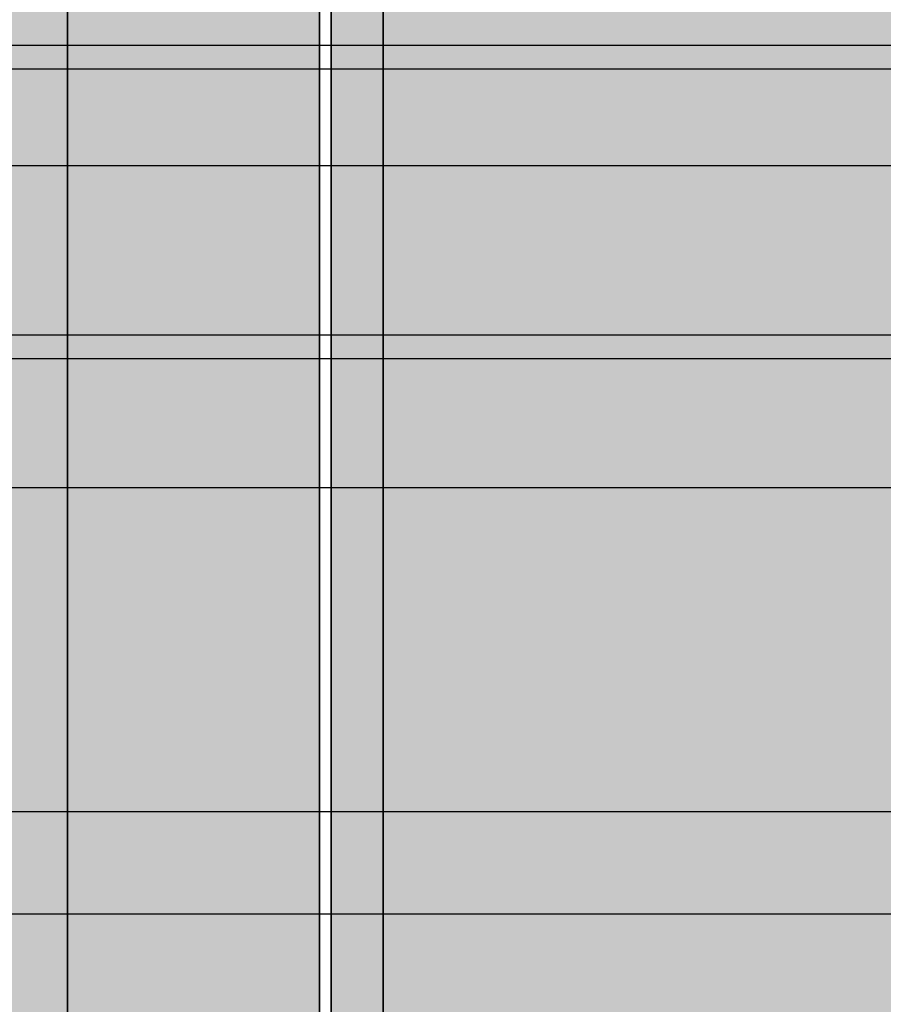
# Model space of a CAD drawing. Units: inches. Extents: x 62 to 566, y 66 to 528.
# Tile 6 of 20: x 138 to 211, y 264 to 347. Entities that reach past the tile are written whole.
import ezdxf

# ---------------------------------------------------------------- set-up
doc = ezdxf.new("R2010")
doc.units = ezdxf.units.IN
doc.header["$MEASUREMENT"] = 0
for name, color, linetype, lineweight in [('A-ANNO-DIMS', 2, 'Continuous', 18), ('A-ELEV', 7, 'Continuous', 35), ('A-WALL-PATT', 8, 'Continuous', 13)]:
    doc.layers.add(name, color=color, linetype=linetype, lineweight=lineweight)
doc.styles.get("Standard").update_dxf_attribs({"font": 'arial.ttf'})
doc.dimstyles.get("Standard").update_dxf_attribs({"dimtxt": 0.75, "dimasz": 0.18, "dimexe": 0.18, "dimexo": 0.0625, "dimgap": 0.09, "dimtad": 0, "dimtih": 1, "dimtoh": 1, "dimdec": 4, "dimzin": 0, "dimdsep": 46, "dimlunit": 4, "dimtxsty": 'Standard', "dimcen": 0.09, "dimadec": 0, "dimazin": 0, "dimtfac": 1, "dimtdec": 4, "dimtofl": 0, "dimtmove": 0, "dimatfit": 3, "dimfxl": 1, "dimtolj": 1, "dimtzin": 0, "dimarcsym": 0})

# ---------------------------------------------------------------- blocks, each defined once
blk = doc.blocks.new('*D8')
at = {"layer": 'A-ANNO-DIMS', "color": 0, "lineweight": -2, "transparency": 16777216}
for p, q in [((284.202, 271.35), (284.202, 65.939)), ((125.942, 126.306), (125.942, 65.939)), ((126.122, 66.119), (203.461, 66.119)), ((284.022, 66.119), (206.683, 66.119))]:
    blk.add_line(p, q, dxfattribs=at)
at = {"layer": 'A-ANNO-DIMS', "color": 0, "transparency": 16777216}
for points in [[(126.122, 66.149), (126.122, 66.089), (125.942, 66.119)], [(284.022, 66.149), (284.022, 66.089), (284.202, 66.119)]]:
    blk.add_solid(points, dxfattribs=at)
at = {"layer": 'Defpoints', "color": 0, "transparency": 16777216}
for p in [(284.202, 271.413), (125.942, 126.369), (284.202, 66.119)]:
    blk.add_point(p, dxfattribs=at)
at = {"layer": 'A-ANNO-DIMS', "color": 0, "transparency": 16777216, "insert": (205.072, 66.119), "char_height": 0.75, "attachment_point": 5}
blk.add_mtext('\\A1;158.26', dxfattribs=at)
blk = doc.blocks.new('*D35')
at = {"layer": 'A-ANNO-DIMS', "color": 0, "lineweight": -2, "transparency": 16777216}
for p, q in [((125.942, 461.98), (125.942, 65.939)), ((142.385, 445.044), (142.385, 65.939)), ((126.122, 66.119), (132.552, 66.119)), ((142.205, 66.119), (135.775, 66.119))]:
    blk.add_line(p, q, dxfattribs=at)
at = {"layer": 'A-ANNO-DIMS', "color": 0, "transparency": 16777216}
for points in [[(126.122, 66.149), (126.122, 66.089), (125.942, 66.119)], [(142.205, 66.149), (142.205, 66.089), (142.385, 66.119)]]:
    blk.add_solid(points, dxfattribs=at)
at = {"layer": 'Defpoints', "color": 0, "transparency": 16777216}
for p in [(125.942, 462.042), (142.385, 445.106), (142.385, 66.119)]:
    blk.add_point(p, dxfattribs=at)
at = {"layer": 'A-ANNO-DIMS', "color": 0, "transparency": 16777216, "insert": (134.163, 66.119), "char_height": 0.75, "attachment_point": 5}
blk.add_mtext('\\A1;16.443', dxfattribs=at)
blk = doc.blocks.new('*D36')
at = {"layer": 'A-ANNO-DIMS', "color": 0, "lineweight": -2, "transparency": 16777216}
for p, q in [((142.385, 445.044), (142.385, 65.939)), ((163.655, 427.413), (163.655, 65.939)), ((142.565, 66.119), (151.658, 66.119)), ((163.475, 66.119), (154.382, 66.119))]:
    blk.add_line(p, q, dxfattribs=at)
at = {"layer": 'A-ANNO-DIMS', "color": 0, "transparency": 16777216}
for points in [[(142.565, 66.149), (142.565, 66.089), (142.385, 66.119)], [(163.475, 66.149), (163.475, 66.089), (163.655, 66.119)]]:
    blk.add_solid(points, dxfattribs=at)
at = {"layer": 'Defpoints', "color": 0, "transparency": 16777216}
for p in [(142.385, 445.106), (163.655, 427.475), (163.655, 66.119)]:
    blk.add_point(p, dxfattribs=at)
at = {"layer": 'A-ANNO-DIMS', "color": 0, "transparency": 16777216, "insert": (153.02, 66.119), "char_height": 0.75, "attachment_point": 5}
blk.add_mtext('\\A1;21.27', dxfattribs=at)
blk = doc.blocks.new('*D37')
at = {"layer": 'A-ANNO-DIMS', "color": 0, "lineweight": -2, "transparency": 16777216}
for p, q in [((163.655, 427.413), (163.655, 65.939)), ((169.043, 420.535), (169.043, 65.939)), ((163.835, 66.119), (164.993, 66.119)), ((168.863, 66.119), (167.705, 66.119))]:
    blk.add_line(p, q, dxfattribs=at)
at = {"layer": 'A-ANNO-DIMS', "color": 0, "transparency": 16777216}
for points in [[(163.835, 66.149), (163.835, 66.089), (163.655, 66.119)], [(168.863, 66.149), (168.863, 66.089), (169.043, 66.119)]]:
    blk.add_solid(points, dxfattribs=at)
at = {"layer": 'Defpoints', "color": 0, "transparency": 16777216}
for p in [(163.655, 427.475), (169.043, 420.597), (169.043, 66.119)]:
    blk.add_point(p, dxfattribs=at)
at = {"layer": 'A-ANNO-DIMS', "color": 0, "transparency": 16777216, "insert": (166.349, 66.119), "char_height": 0.75, "attachment_point": 5}
blk.add_mtext('\\A1;5.388', dxfattribs=at)
blk = doc.blocks.new('*D38')
at = {"layer": 'A-ANNO-DIMS', "color": 0, "lineweight": -2, "transparency": 16777216}
for p, q in [((169.043, 420.535), (169.043, 65.939)), ((217.275, 420.535), (217.275, 65.939)), ((169.223, 66.119), (191.789, 66.119)), ((217.095, 66.119), (194.53, 66.119))]:
    blk.add_line(p, q, dxfattribs=at)
at = {"layer": 'A-ANNO-DIMS', "color": 0, "transparency": 16777216}
for points in [[(169.223, 66.149), (169.223, 66.089), (169.043, 66.119)], [(217.095, 66.149), (217.095, 66.089), (217.275, 66.119)]]:
    blk.add_solid(points, dxfattribs=at)
at = {"layer": 'Defpoints', "color": 0, "transparency": 16777216}
for p in [(169.043, 420.597), (217.275, 420.597), (217.275, 66.119)]:
    blk.add_point(p, dxfattribs=at)
at = {"layer": 'A-ANNO-DIMS', "color": 0, "transparency": 16777216, "insert": (193.159, 66.119), "char_height": 0.75, "attachment_point": 5}
blk.add_mtext('\\A1;48.23', dxfattribs=at)
blk = doc.blocks.new('*D98')
at = {"layer": 'A-ANNO-DIMS', "color": 0, "lineweight": -2, "transparency": 16777216}
for p, q in [((296.313, 280.042), (63.466, 280.042)), ((63.646, 279.862), (63.646, 276.201)), ((63.646, 271.593), (63.646, 275.254)), ((284.14, 271.413), (63.466, 271.413))]:
    blk.add_line(p, q, dxfattribs=at)
at = {"layer": 'A-ANNO-DIMS', "color": 0, "transparency": 16777216}
for points in [[(63.616, 279.862), (63.676, 279.862), (63.646, 280.042)], [(63.616, 271.593), (63.676, 271.593), (63.646, 271.413)]]:
    blk.add_solid(points, dxfattribs=at)
at = {"layer": 'Defpoints', "color": 0, "transparency": 16777216}
for p in [(63.646, 280.042), (296.375, 280.042), (284.202, 271.413)]:
    blk.add_point(p, dxfattribs=at)
at = {"layer": 'A-ANNO-DIMS', "color": 0, "transparency": 16777216, "insert": (63.646, 275.728), "char_height": 0.75, "attachment_point": 5}
blk.add_mtext('\\A1;8.63', dxfattribs=at)
blk = doc.blocks.new('*D99')
at = {"layer": 'A-ANNO-DIMS', "color": 0, "lineweight": -2, "transparency": 16777216}
for p, q in [((284.14, 318.305), (63.466, 318.305)), ((63.646, 318.125), (63.646, 313.332)), ((63.646, 307.593), (63.646, 312.386)), ((284.14, 307.413), (63.466, 307.413))]:
    blk.add_line(p, q, dxfattribs=at)
at = {"layer": 'A-ANNO-DIMS', "color": 0, "transparency": 16777216}
for points in [[(63.616, 318.125), (63.676, 318.125), (63.646, 318.305)], [(63.616, 307.593), (63.676, 307.593), (63.646, 307.413)]]:
    blk.add_solid(points, dxfattribs=at)
at = {"layer": 'Defpoints', "color": 0, "transparency": 16777216}
for p in [(63.646, 318.305), (284.202, 318.305), (284.202, 307.413)]:
    blk.add_point(p, dxfattribs=at)
at = {"layer": 'A-ANNO-DIMS', "color": 0, "transparency": 16777216, "insert": (63.646, 312.859), "char_height": 0.75, "attachment_point": 5}
blk.add_mtext('\\A1;10.892', dxfattribs=at)
blk = doc.blocks.new('*D100')
at = {"layer": 'A-ANNO-DIMS', "color": 0, "lineweight": -2, "transparency": 16777216}
for p, q in [((284.14, 334.612), (63.466, 334.612)), ((63.646, 334.432), (63.646, 326.932)), ((63.646, 318.485), (63.646, 325.985)), ((284.14, 318.305), (63.466, 318.305))]:
    blk.add_line(p, q, dxfattribs=at)
at = {"layer": 'A-ANNO-DIMS', "color": 0, "transparency": 16777216}
for points in [[(63.616, 334.432), (63.676, 334.432), (63.646, 334.612)], [(63.616, 318.485), (63.676, 318.485), (63.646, 318.305)]]:
    blk.add_solid(points, dxfattribs=at)
at = {"layer": 'Defpoints', "color": 0, "transparency": 16777216}
for p in [(63.646, 334.612), (284.202, 334.612), (284.202, 318.305)]:
    blk.add_point(p, dxfattribs=at)
at = {"layer": 'A-ANNO-DIMS', "color": 0, "transparency": 16777216, "insert": (63.646, 326.458), "char_height": 0.75, "attachment_point": 5}
blk.add_mtext('\\A1;16.307', dxfattribs=at)
blk = doc.blocks.new('*D101')
at = {"layer": 'A-ANNO-DIMS', "color": 0, "lineweight": -2, "transparency": 16777216}
for p, q in [((284.14, 342.782), (63.466, 342.782)), ((63.646, 342.602), (63.646, 339.17)), ((63.646, 334.792), (63.646, 338.224)), ((284.14, 334.612), (63.466, 334.612))]:
    blk.add_line(p, q, dxfattribs=at)
at = {"layer": 'A-ANNO-DIMS', "color": 0, "transparency": 16777216}
for points in [[(63.616, 342.602), (63.676, 342.602), (63.646, 342.782)], [(63.616, 334.792), (63.676, 334.792), (63.646, 334.612)]]:
    blk.add_solid(points, dxfattribs=at)
at = {"layer": 'Defpoints', "color": 0, "transparency": 16777216}
for p in [(63.646, 342.782), (284.202, 342.782), (284.202, 334.612)]:
    blk.add_point(p, dxfattribs=at)
at = {"layer": 'A-ANNO-DIMS', "color": 0, "transparency": 16777216, "insert": (63.646, 338.697), "char_height": 0.75, "attachment_point": 5}
blk.add_mtext('\\A1;8.17', dxfattribs=at)
blk = doc.blocks.new('*D102')
at = {"layer": 'A-ANNO-DIMS', "color": 0, "lineweight": -2, "transparency": 16777216}
for p, q in [((284.14, 344.782), (63.466, 344.782)), ((63.646, 344.602), (63.646, 344.249)), ((284.14, 342.782), (63.466, 342.782)), ((63.646, 342.962), (63.646, 343.316))]:
    blk.add_line(p, q, dxfattribs=at)
at = {"layer": 'A-ANNO-DIMS', "color": 0, "transparency": 16777216}
for points in [[(63.616, 344.602), (63.676, 344.602), (63.646, 344.782)], [(63.616, 342.962), (63.676, 342.962), (63.646, 342.782)]]:
    blk.add_solid(points, dxfattribs=at)
at = {"layer": 'Defpoints', "color": 0, "transparency": 16777216}
for p in [(63.646, 344.782), (284.202, 344.782), (284.202, 342.782)]:
    blk.add_point(p, dxfattribs=at)
at = {"layer": 'A-ANNO-DIMS', "color": 0, "transparency": 16777216, "insert": (63.646, 343.782), "char_height": 0.75, "attachment_point": 5}
blk.add_mtext('\\A1;2', dxfattribs=at)
blk = doc.blocks.new('*D103')
at = {"layer": 'A-ANNO-DIMS', "color": 0, "lineweight": -2, "transparency": 16777216}
for p, q in [((284.14, 320.305), (63.466, 320.305)), ((63.646, 320.125), (63.646, 319.772)), ((63.646, 318.485), (63.646, 318.839)), ((284.14, 318.305), (63.466, 318.305))]:
    blk.add_line(p, q, dxfattribs=at)
at = {"layer": 'A-ANNO-DIMS', "color": 0, "transparency": 16777216}
for points in [[(63.616, 320.125), (63.676, 320.125), (63.646, 320.305)], [(63.616, 318.485), (63.676, 318.485), (63.646, 318.305)]]:
    blk.add_solid(points, dxfattribs=at)
at = {"layer": 'Defpoints', "color": 0, "transparency": 16777216}
for p in [(63.646, 320.305), (284.202, 320.305), (284.202, 318.305)]:
    blk.add_point(p, dxfattribs=at)
at = {"layer": 'A-ANNO-DIMS', "color": 0, "transparency": 16777216, "insert": (63.646, 319.305), "char_height": 0.75, "attachment_point": 5}
blk.add_mtext('\\A1;2', dxfattribs=at)
blk = doc.blocks.new('*D130')
at = {"layer": 'A-ANNO-DIMS', "color": 0, "lineweight": -2, "transparency": 16777216}
for p, q in [((227.738, 280.042), (63.466, 280.042)), ((63.646, 279.862), (63.646, 276.201)), ((63.646, 271.593), (63.646, 275.254)), ((217.213, 271.413), (63.466, 271.413))]:
    blk.add_line(p, q, dxfattribs=at)
at = {"layer": 'A-ANNO-DIMS', "color": 0, "transparency": 16777216}
for points in [[(63.616, 279.862), (63.676, 279.862), (63.646, 280.042)], [(63.616, 271.593), (63.676, 271.593), (63.646, 271.413)]]:
    blk.add_solid(points, dxfattribs=at)
at = {"layer": 'Defpoints', "color": 0, "transparency": 16777216}
for p in [(63.646, 280.042), (227.8, 280.042), (217.275, 271.413)]:
    blk.add_point(p, dxfattribs=at)
at = {"layer": 'A-ANNO-DIMS', "color": 0, "transparency": 16777216, "insert": (63.646, 275.728), "char_height": 0.75, "attachment_point": 5}
blk.add_mtext('\\A1;8.63', dxfattribs=at)

msp = doc.modelspace()

# ---------------------------------------------------------------- hatches: boundary and pattern name
at = {"layer": 'A-WALL-PATT'}
h = msp.add_hatch(color=256, dxfattribs=at)
h.dxf.hatch_style = 1
h.paths.add_polyline_path([(416.0836, 462.0423), (125.9418, 462.0423), (125.9418, 414.3686), (125.9418, 270.3686), (125.9418, 126.3686), (142.3851, 126.3686), (142.3851, 270.3686), (142.3851, 414.3686), (142.3851, 445.1064), (284.2021, 445.1064), (416.0836, 445.1064)])
h.paths.add_polyline_path([(435.3945, 503.0423), (426.3652, 503.0423), (120.4058, 503.0423), (120.4058, 501.0423), (125.9418, 501.0423), (416.0836, 501.0423), (426.3652, 501.0423), (430.6938, 501.0423), (435.3945, 501.0423)])
h.paths.add_polyline_path([(439.6878, 352.4848), (392.4793, 352.4848), (392.4793, 307.4128), (217.2752, 307.4128), (217.2752, 295.4098), (217.2752, 271.4128), (272.0586, 271.4128), (439.6878, 271.4128)])
h.paths.add_polyline_path([(248.0143, 297.1682), (255.6783, 297.1682), (255.6783, 280.0423), (248.0143, 280.0423)], flags=16)
h.paths.add_polyline_path([(235.4641, 280.0423), (227.8001, 280.0423), (227.8001, 297.1682), (235.4641, 297.1682)], flags=16)
h.paths.add_polyline_path([(270.4427, 297.1682), (278.1067, 297.1682), (278.1067, 280.0423), (270.4427, 280.0423)], flags=16)
h.paths.add_polyline_path([(296.3755, 297.1682), (304.0395, 297.1682), (304.0395, 280.0423), (296.3755, 280.0423)], flags=16)
h.paths.add_polyline_path([(319.2543, 297.1682), (326.9183, 297.1682), (326.9183, 280.0423), (319.2543, 280.0423)], flags=16)
h.paths.add_polyline_path([(341.2622, 297.1682), (348.9262, 297.1682), (348.9262, 280.0423), (341.2622, 280.0423)], flags=16)
h.paths.add_polyline_path([(389.2857, 298.3985), (433.8102, 298.3985), (433.8102, 294.9497), (389.2857, 294.9497)], flags=16)
h.paths.add_polyline_path([(389.2857, 291.6038), (433.8102, 291.6038), (433.8102, 288.155), (389.2857, 288.155)], flags=16)
h.paths.add_polyline_path([(389.2857, 284.9607), (433.8102, 284.9607), (433.8102, 281.5119), (389.2857, 281.5119)], flags=16)
h.paths.add_polyline_path([(403.5849, 311.4736), (403.5849, 317.4388), (433.1636, 317.4388), (433.1636, 311.4736)], flags=16)
h.paths.add_polyline_path([(403.5849, 323.1329), (403.5849, 329.0982), (433.1636, 329.0982), (433.1636, 323.1329)], flags=16)
h.paths.add_polyline_path([(403.5849, 334.5211), (403.5849, 340.4863), (433.1636, 340.4863), (433.1636, 334.5211)], flags=16)
h.paths.add_polyline_path([(272.0586, 160.3545), (217.2752, 160.3545), (217.2752, 129.0504), (217.2752, 126.3686), (272.0586, 126.3686)], flags=17)
h.paths.add_polyline_path([(220.5897, 149.5749), (220.5897, 152.296), (267.7931, 152.296), (267.7931, 149.5749)], flags=16)
h.paths.add_polyline_path([(267.7931, 146.6724), (267.7931, 143.9513), (220.5897, 143.9513), (220.5897, 146.6724)], flags=16)
h.paths.add_polyline_path([(220.5897, 155.3799), (220.5897, 158.101), (267.7931, 158.101), (267.7931, 155.3799)], flags=16)
h.paths.add_polyline_path([(267.7931, 140.686), (267.7931, 137.9649), (220.5897, 137.9649), (220.5897, 140.686)], flags=16)
h.paths.add_polyline_path([(267.7931, 135.516), (267.7931, 132.7949), (220.5897, 132.7949), (220.5897, 135.516)], flags=16)
h = msp.add_hatch(dxfattribs=at)
h.set_pattern_fill('ANSI36', color=256, scale=8.8)
h.paths.add_polyline_path([(217.2752, 420.597), (169.0431, 420.597), (169.0431, 126.3686), (217.2752, 126.3686), (217.2752, 129.0504), (217.2752, 271.4128), (217.2752, 295.4128), (217.2752, 307.4128)])
h.paths.add_polyline_path([(282.3509, 501.0423), (125.9418, 501.0423), (125.9418, 465.0423), (282.3509, 465.0423)])
h.paths.add_polyline_path([(209.709, 476.6506), (202.045, 476.6506), (202.045, 493.7764), (209.709, 493.7764)], flags=16)
h.paths.add_polyline_path([(193.9913, 476.6506), (186.3273, 476.6506), (186.3273, 493.7764), (193.9913, 493.7764)], flags=16)
h.paths.add_polyline_path([(177.9243, 476.6506), (170.2603, 476.6506), (170.2603, 493.7764), (177.9243, 493.7764)], flags=16)
h.paths.add_polyline_path([(163.2545, 476.3015), (155.5905, 476.3015), (155.5905, 493.4274), (163.2545, 493.4274)], flags=16)
h.paths.add_polyline_path([(148.2354, 476.3015), (140.5713, 476.3015), (140.5713, 493.4274), (148.2354, 493.4274)], flags=16)
h.paths.add_polyline_path([(284.2021, 126.3686), (87.8962, 126.3686), (87.8962, 114.3686), (87.8962, 90.3686), (284.2021, 90.3686)])
h.paths.add_polyline_path([(474.1214, 126.3686), (396.433, 126.3686), (396.433, 90.3686), (474.1214, 90.3686)])
h = msp.add_hatch(color=256, dxfattribs=at)
h.dxf.hatch_style = 1
h.paths.add_polyline_path([(416.0836, 501.0423), (282.3509, 501.0423), (282.3509, 465.0423), (416.0836, 465.0423)])
h.paths.add_polyline_path([(284.2021, 420.597), (272.0586, 420.597), (272.0586, 309.5388), (272.0586, 307.4128), (284.2021, 307.4128)], flags=17)
h.paths.add_polyline_path([(284.2021, 445.1064), (142.3851, 445.1064), (142.3851, 414.3686), (142.3851, 270.3686), (142.3851, 126.3686), (163.6548, 126.3686), (163.6548, 270.5016), (163.6548, 414.5016), (163.6548, 427.4752), (284.2021, 427.4752)])
h.paths.add_polyline_path([(235.4641, 297.1682), (227.8001, 297.1682), (227.8001, 280.0423), (235.4641, 280.0423)], flags=17)
h.paths.add_polyline_path([(255.6783, 297.1682), (248.0143, 297.1682), (248.0143, 280.0423), (255.6783, 280.0423)], flags=17)
h.paths.add_polyline_path([(278.1067, 297.1682), (270.4427, 297.1682), (270.4427, 280.0423), (278.1067, 280.0423)], flags=17)
h.paths.add_polyline_path([(304.0395, 297.1682), (296.3755, 297.1682), (296.3755, 280.0423), (304.0395, 280.0423)])
h.paths.add_polyline_path([(326.9183, 297.1682), (319.2543, 297.1682), (319.2543, 280.0423), (326.9183, 280.0423)])
h.paths.add_polyline_path([(348.9262, 297.1682), (341.2622, 297.1682), (341.2622, 280.0423), (348.9262, 280.0423)])
h.paths.add_polyline_path([(433.8102, 284.9607), (389.2857, 284.9607), (389.2857, 281.5119), (433.8102, 281.5119)])
h.paths.add_polyline_path([(433.8102, 291.6038), (389.2857, 291.6038), (389.2857, 288.155), (433.8102, 288.155)])
h.paths.add_polyline_path([(433.8102, 298.3985), (389.2857, 298.3985), (389.2857, 294.9497), (433.8102, 294.9497)])
h.paths.add_polyline_path([(433.1636, 317.4388), (403.5849, 317.4388), (403.5849, 311.4736), (433.1636, 311.4736)])
h.paths.add_polyline_path([(433.1636, 329.0982), (403.5849, 329.0982), (403.5849, 323.1329), (433.1636, 323.1329)])
h.paths.add_polyline_path([(433.1636, 340.4863), (403.5849, 340.4863), (403.5849, 334.5211), (433.1636, 334.5211)])
h.paths.add_polyline_path([(284.2021, 271.4128), (272.0586, 271.4128), (272.0586, 160.3545), (272.0586, 126.3686), (284.2021, 126.3686)])
h.paths.add_polyline_path([(267.7931, 158.101), (220.5897, 158.101), (220.5897, 155.3799), (267.7931, 155.3799)], flags=17)
h.paths.add_polyline_path([(267.7931, 152.296), (220.5897, 152.296), (220.5897, 149.5749), (267.7931, 149.5749)], flags=17)
h.paths.add_polyline_path([(267.7931, 146.6724), (220.5897, 146.6724), (220.5897, 143.9513), (267.7931, 143.9513)], flags=17)
h.paths.add_polyline_path([(267.7931, 140.686), (220.5897, 140.686), (220.5897, 137.9649), (267.7931, 137.9649)], flags=17)
h.paths.add_polyline_path([(267.7931, 135.516), (220.5897, 135.516), (220.5897, 132.7949), (267.7931, 132.7949)], flags=17)
h.paths.add_polyline_path([(148.2354, 493.4274), (140.5713, 493.4274), (140.5713, 476.3015), (148.2354, 476.3015)])
h.paths.add_polyline_path([(163.2545, 493.4274), (155.5905, 493.4274), (155.5905, 476.3015), (163.2545, 476.3015)])
h.paths.add_polyline_path([(177.9243, 493.7764), (170.2603, 493.7764), (170.2603, 476.6506), (177.9243, 476.6506)])
h.paths.add_polyline_path([(193.9913, 493.7764), (186.3273, 493.7764), (186.3273, 476.6506), (193.9913, 476.6506)])
h.paths.add_polyline_path([(209.709, 493.7764), (202.045, 493.7764), (202.045, 476.6506), (209.709, 476.6506)])
h = msp.add_hatch(color=256, dxfattribs=at)
h.dxf.hatch_style = 1
h.paths.add_polyline_path([(430.6938, 462.0423), (416.0836, 462.0423), (416.0836, 445.1064), (430.6938, 445.1064)])
h.paths.add_polyline_path([(169.0431, 420.597), (284.2021, 420.597), (284.2021, 426.4752), (164.6548, 426.4752), (164.6548, 414.5016), (164.6548, 126.3686), (169.0431, 126.3686)])

# ---------------------------------------------------------------- linework, layer by layer
at = {"layer": 'A-ELEV'}
for p, q in [((169.0431, 126.3686), (169.0431, 420.597)), ((142.3851, 270.3686), (142.3851, 414.3686)), ((142.3851, 126.3686), (142.3851, 270.3686))]:
    msp.add_line(p, q, dxfattribs=at)
for points in [[(163.6548, 126.3686), (163.6548, 414.5016), (163.6548, 427.4752), (284.2021, 427.4752)], [(164.6548, 126.3686), (164.6548, 414.5016), (164.6548, 426.4752), (284.2021, 426.4752)]]:
    msp.add_lwpolyline(points, dxfattribs=at)

# ---------------------------------------------------------------- dimensions: what is measured, and where the dimension line sits
at = {"layer": 'A-ANNO-DIMS'}
for base, p1, p2, override, picture, middle in [((142.3851, 66.1186), (125.9418, 462.0423), (142.3851, 445.1064), {"dimdec": 3, "dimlfac": 1, "dimrnd": 0, "dimzin": 0, "dimdsep": 46, "dimlunit": 2}, '*D35', (134.1634, 66.1186)), ((163.6548, 66.1186), (142.3851, 445.1064), (163.6548, 427.4752), {"dimdec": 2, "dimlfac": 1, "dimrnd": 0, "dimzin": 0, "dimdsep": 46, "dimlunit": 2}, '*D36', (153.0199, 66.1186)), ((169.0431, 66.1186), (163.6548, 427.4752), (169.0431, 420.597), {"dimdec": 3, "dimlfac": 1, "dimrnd": 0, "dimzin": 0, "dimdsep": 46, "dimlunit": 2}, '*D37', (166.349, 66.1186)), ((217.2752, 66.1186), (169.0431, 420.597), (217.2752, 420.597), {"dimdec": 2, "dimlfac": 1, "dimrnd": 0, "dimzin": 0, "dimdsep": 46, "dimlunit": 2}, '*D38', (193.1592, 66.1186)), ((284.2021, 66.1186), (125.9418, 126.3686), (284.2021, 271.4128), {"dimdec": 2, "dimlfac": 1, "dimrnd": 0, "dimzin": 0, "dimdsep": 46, "dimlunit": 2}, '*D8', (205.0719, 66.1186))]:
    dim = msp.add_linear_dim(base=base, p1=p1, p2=p2, dimstyle='Standard', override=override, dxfattribs=at)
    dim.commit()
    dim.dimension.update_dxf_attribs({"geometry": picture, "text_midpoint": middle})
for base, p1, p2, override, picture, middle in [((63.6462, 344.7821), (284.2021, 342.7821), (284.2021, 344.7821), {"dimdec": 0, "dimlfac": 1, "dimrnd": 0, "dimzin": 0, "dimdsep": 46, "dimlunit": 2}, '*D102', (63.6462, 343.7821)), ((63.6462, 342.7821), (284.2021, 334.6119), (284.2021, 342.7821), {"dimdec": 2, "dimlfac": 1, "dimrnd": 0, "dimzin": 0, "dimdsep": 46, "dimlunit": 2}, '*D101', (63.6462, 338.697)), ((63.6462, 334.6119), (284.2021, 318.3051), (284.2021, 334.6119), {"dimdec": 3, "dimlfac": 1, "dimrnd": 0, "dimzin": 0, "dimdsep": 46, "dimlunit": 2}, '*D100', (63.6462, 326.4585)), ((63.6462, 320.3051), (284.2021, 318.3051), (284.2021, 320.3051), {"dimdec": 0, "dimlfac": 1, "dimrnd": 0, "dimzin": 0, "dimdsep": 46, "dimlunit": 2}, '*D103', (63.6462, 319.3051)), ((63.6462, 318.3051), (284.2021, 307.4128), (284.2021, 318.3051), {"dimdec": 3, "dimlfac": 1, "dimrnd": 0, "dimzin": 0, "dimdsep": 46, "dimlunit": 2}, '*D99', (63.6462, 312.8589)), ((63.6462, 280.0423), (284.2021, 271.4128), (296.3755, 280.0423), {"dimdec": 2, "dimlfac": 1, "dimrnd": 0, "dimzin": 0, "dimdsep": 46, "dimlunit": 2}, '*D98', (63.6462, 275.7276)), ((63.6462, 280.0423), (217.2752, 271.4128), (227.8001, 280.0423), {"dimdec": 2, "dimlfac": 1, "dimrnd": 0, "dimzin": 0, "dimdsep": 46, "dimlunit": 2}, '*D130', (63.6462, 275.7276))]:
    dim = msp.add_linear_dim(base=base, p1=p1, p2=p2, angle=90, dimstyle='Standard', override=override, dxfattribs=at)
    dim.commit()
    dim.dimension.update_dxf_attribs({"geometry": picture, "text_midpoint": middle})

doc.saveas('drawing.dxf')
